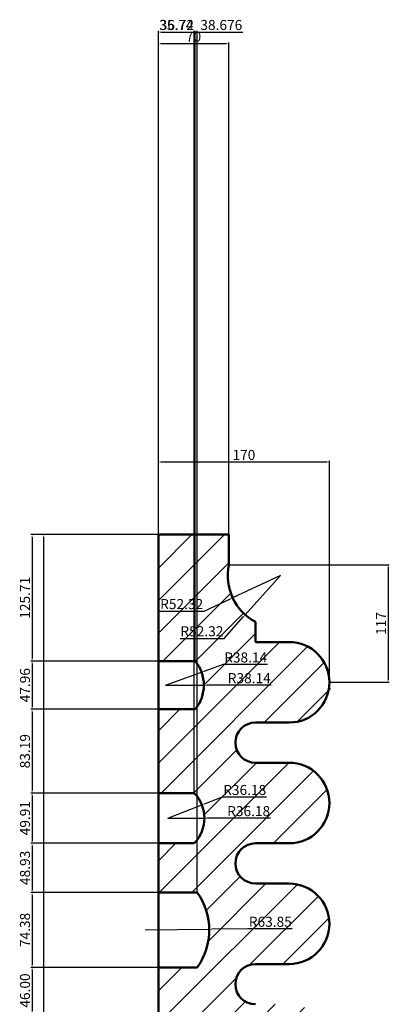
# Model space of a CAD drawing. Units: millimetres. Extents: x 1178 to 3717, y 924 to 2764.
# Tile 3 of 5: x 1208 to 1576, y 1785 to 2764. Entities that reach past the tile are written whole.
import ezdxf

# ---------------------------------------------------------------- set-up
doc = ezdxf.new("R2010")
doc.units = ezdxf.units.MM
for name, color, linetype, lineweight in [('M-DIMS', 2, 'Continuous', 25), ('M-HATC', 8, 'Continuous', 18), ('M-OUTL', 7, 'Continuous', 50)]:
    doc.layers.add(name, color=color, linetype=linetype, lineweight=lineweight)
doc.styles.get("Standard").update_dxf_attribs({"font": 'arial.ttf'})
doc.dimstyles.new('ISO-25', dxfattribs={"dimtxt": 10, "dimasz": 2.5, "dimexe": 1.25, "dimexo": 0.625, "dimtad": 1, "dimtoh": 1, "dimdec": 0, "dimtxsty": 'Standard', "dimcen": 2.5, "dimadec": 0, "dimazin": 0, "dimtfac": 1, "dimtdec": 0, "dimtmove": 0, "dimatfit": 3, "dimfxl": 1, "dimarcsym": 0})

# ---------------------------------------------------------------- blocks, each defined once
blk = doc.blocks.new('*D24')
at = {"layer": 'Defpoints', "color": 0, "transparency": 16777216}
for p in [(1516.06, 2324.34), (1346.06, 2252.21), (1516.06, 2099.53)]:
    blk.add_point(p, dxfattribs=at)
at = {"layer": 'M-DIMS', "color": 0, "lineweight": -2, "transparency": 16777216}
for p, q in [((1346.06, 2252.84), (1346.06, 2325.59)), ((1348.56, 2324.34), (1513.56, 2324.34)), ((1516.06, 2100.16), (1516.06, 2325.59))]:
    blk.add_line(p, q, dxfattribs=at)
at = {"layer": 'M-DIMS', "color": 0, "transparency": 16777216}
for points in [[(1348.56, 2324.76), (1348.56, 2323.93), (1346.06, 2324.34)], [(1513.56, 2324.76), (1513.56, 2323.93), (1516.06, 2324.34)]]:
    blk.add_solid(points, dxfattribs=at)
at = {"layer": 'M-DIMS', "color": 0, "transparency": 16777216, "insert": (1431.06, 2330.07), "char_height": 10, "attachment_point": 5}
blk.add_mtext('170', dxfattribs=at)
blk = doc.blocks.new('*D25')
at = {"layer": 'Defpoints', "color": 0, "transparency": 16777216}
for p in [(1416.06, 2222.21), (1516.07, 2105.43), (1574.3, 2105.43)]:
    blk.add_point(p, dxfattribs=at)
at = {"layer": 'M-DIMS', "color": 0, "lineweight": -2, "transparency": 16777216}
for p, q in [((1416.69, 2222.21), (1575.55, 2222.21)), ((1574.3, 2219.71), (1574.3, 2107.93)), ((1516.69, 2105.43), (1575.55, 2105.43))]:
    blk.add_line(p, q, dxfattribs=at)
at = {"layer": 'M-DIMS', "color": 0, "transparency": 16777216}
for points in [[(1573.89, 2219.71), (1574.72, 2219.71), (1574.3, 2222.21)], [(1573.89, 2107.93), (1574.72, 2107.93), (1574.3, 2105.43)]]:
    blk.add_solid(points, dxfattribs=at)
at = {"layer": 'M-DIMS', "color": 0, "transparency": 16777216, "insert": (1568.66, 2163.82), "char_height": 10, "attachment_point": 5, "rotation": 90}
blk.add_mtext('117', dxfattribs=at)
blk = doc.blocks.new('*D49')
at = {"layer": 'Defpoints', "color": 0, "transparency": 16777216}
for p in [(1346.06, 2252.21), (1232.06, 1051.02), (1346.06, 1051.02)]:
    blk.add_point(p, dxfattribs=at)
at = {"layer": 'M-DIMS', "color": 0, "lineweight": -2, "transparency": 16777216}
for p, q in [((1345.44, 2252.21), (1230.81, 2252.21)), ((1232.06, 2249.71), (1232.06, 1053.52)), ((1345.44, 1051.02), (1230.81, 1051.02))]:
    blk.add_line(p, q, dxfattribs=at)
at = {"layer": 'M-DIMS', "color": 0, "transparency": 16777216}
for points in [[(1231.64, 2249.71), (1232.48, 2249.71), (1232.06, 2252.21)], [(1231.64, 1053.52), (1232.48, 1053.52), (1232.06, 1051.02)]]:
    blk.add_solid(points, dxfattribs=at)
at = {"layer": 'M-DIMS', "color": 0, "transparency": 16777216, "insert": (1226.33, 1651.62), "char_height": 10, "attachment_point": 5, "rotation": 90}
blk.add_mtext('1201.2', dxfattribs=at)
blk = doc.blocks.new('*D50')
at = {"layer": 'Defpoints', "color": 0, "transparency": 16777216}
for p in [(1416.06, 2740.04), (1346.06, 2252.21), (1416.06, 2222.21)]:
    blk.add_point(p, dxfattribs=at)
at = {"layer": 'M-DIMS', "color": 0, "lineweight": -2, "transparency": 16777216}
for p, q in [((1346.06, 2252.84), (1346.06, 2741.29)), ((1348.56, 2740.04), (1413.56, 2740.04)), ((1416.06, 2222.84), (1416.06, 2741.29))]:
    blk.add_line(p, q, dxfattribs=at)
at = {"layer": 'M-DIMS', "color": 0, "transparency": 16777216}
for points in [[(1348.56, 2740.46), (1348.56, 2739.62), (1346.06, 2740.04)], [(1413.56, 2740.46), (1413.56, 2739.62), (1416.06, 2740.04)]]:
    blk.add_solid(points, dxfattribs=at)
at = {"layer": 'M-DIMS', "color": 0, "transparency": 16777216, "insert": (1381.06, 2745.77), "char_height": 10, "attachment_point": 5}
blk.add_mtext('70', dxfattribs=at)
blk = doc.blocks.new('*D60')
at = {"layer": 'Defpoints', "color": 0, "transparency": 16777216}
for p in [(1467.29, 2211.56), (1419.89, 2189.4)]:
    blk.add_point(p, dxfattribs=at)
at = {"layer": 'M-DIMS', "color": 0, "lineweight": -2, "transparency": 16777216}
for p, q in [((1467.29, 2211.56), (1419.89, 2189.4)), ((1391.46, 2176.1), (1417.63, 2188.34)), ((1347.62, 2176.1), (1391.46, 2176.1))]:
    blk.add_line(p, q, dxfattribs=at)
at = {"layer": 'M-DIMS', "color": 0, "transparency": 16777216}
blk.add_solid([(1417.45, 2188.72), (1417.81, 2187.96), (1419.89, 2189.4)], dxfattribs=at)
at = {"layer": 'M-DIMS', "color": 0, "transparency": 16777216, "insert": (1369.22, 2181.83), "char_height": 10, "attachment_point": 5}
blk.add_mtext('R52.32', dxfattribs=at)
blk = doc.blocks.new('*D63')
at = {"layer": 'Defpoints', "color": 0, "transparency": 16777216}
for p in [(1353.12, 2102.53), (1391.26, 2102.5)]:
    blk.add_point(p, dxfattribs=at)
at = {"layer": 'M-DIMS', "color": 0, "lineweight": -2, "transparency": 16777216}
for p, q in [((1353.12, 2102.53), (1391.26, 2102.5)), ((1414.14, 2102.48), (1393.76, 2102.5)), ((1458.04, 2102.48), (1414.14, 2102.48))]:
    blk.add_line(p, q, dxfattribs=at)
at = {"layer": 'M-DIMS', "color": 0, "transparency": 16777216}
blk.add_solid([(1393.76, 2102.91), (1393.76, 2102.08), (1391.26, 2102.5)], dxfattribs=at)
at = {"layer": 'M-DIMS', "color": 0, "transparency": 16777216, "insert": (1436.4, 2108.22), "char_height": 10, "attachment_point": 5}
blk.add_mtext('R38.14', dxfattribs=at)
blk = doc.blocks.new('*D64')
at = {"layer": 'Defpoints', "color": 0, "transparency": 16777216}
for p in [(1355.6, 1970.4), (1391.78, 1970.4)]:
    blk.add_point(p, dxfattribs=at)
at = {"layer": 'M-DIMS', "color": 0, "lineweight": -2, "transparency": 16777216}
for p, q in [((1355.6, 1970.4), (1391.78, 1970.4)), ((1413.49, 1970.4), (1394.28, 1970.4)), ((1457.45, 1970.4), (1413.49, 1970.4))]:
    blk.add_line(p, q, dxfattribs=at)
at = {"layer": 'M-DIMS', "color": 0, "transparency": 16777216}
blk.add_solid([(1394.28, 1970.82), (1394.28, 1969.98), (1391.78, 1970.4)], dxfattribs=at)
at = {"layer": 'M-DIMS', "color": 0, "transparency": 16777216, "insert": (1435.78, 1976.13), "char_height": 10, "attachment_point": 5}
blk.add_mtext('R36.18', dxfattribs=at)
blk = doc.blocks.new('*D72')
at = {"layer": 'Defpoints', "color": 0, "transparency": 16777216}
for p in [(1346.06, 2252.21), (1220.56, 2126.5), (1346.06, 2126.5)]:
    blk.add_point(p, dxfattribs=at)
at = {"layer": 'M-DIMS', "color": 0, "lineweight": -2, "transparency": 16777216}
for p, q in [((1345.44, 2252.21), (1219.31, 2252.21)), ((1220.56, 2249.71), (1220.56, 2129)), ((1345.44, 2126.5), (1219.31, 2126.5))]:
    blk.add_line(p, q, dxfattribs=at)
at = {"layer": 'M-DIMS', "color": 0, "transparency": 16777216}
for points in [[(1220.14, 2249.71), (1220.98, 2249.71), (1220.56, 2252.21)], [(1220.14, 2129), (1220.98, 2129), (1220.56, 2126.5)]]:
    blk.add_solid(points, dxfattribs=at)
at = {"layer": 'M-DIMS', "color": 0, "transparency": 16777216, "insert": (1214.83, 2189.36), "char_height": 10, "attachment_point": 5, "rotation": 90}
blk.add_mtext('125.71', dxfattribs=at)
blk = doc.blocks.new('*D73')
at = {"layer": 'Defpoints', "color": 0, "transparency": 16777216}
for p in [(1346.06, 2126.5), (1220.56, 2078.55), (1346.06, 2078.55)]:
    blk.add_point(p, dxfattribs=at)
at = {"layer": 'M-DIMS', "color": 0, "lineweight": -2, "transparency": 16777216}
for p, q in [((1345.44, 2126.5), (1219.31, 2126.5)), ((1220.56, 2124), (1220.56, 2081.05)), ((1345.44, 2078.55), (1219.31, 2078.55))]:
    blk.add_line(p, q, dxfattribs=at)
at = {"layer": 'M-DIMS', "color": 0, "transparency": 16777216}
for points in [[(1220.14, 2124), (1220.98, 2124), (1220.56, 2126.5)], [(1220.14, 2081.05), (1220.98, 2081.05), (1220.56, 2078.55)]]:
    blk.add_solid(points, dxfattribs=at)
at = {"layer": 'M-DIMS', "color": 0, "transparency": 16777216, "insert": (1214.83, 2102.53), "char_height": 10, "attachment_point": 5, "rotation": 90}
blk.add_mtext('47.96', dxfattribs=at)
blk = doc.blocks.new('*D74')
at = {"layer": 'Defpoints', "color": 0, "transparency": 16777216}
for p in [(1346.06, 2078.55), (1220.56, 1995.36), (1346.06, 1995.36)]:
    blk.add_point(p, dxfattribs=at)
at = {"layer": 'M-DIMS', "color": 0, "lineweight": -2, "transparency": 16777216}
for p, q in [((1345.44, 2078.55), (1219.31, 2078.55)), ((1220.56, 2076.05), (1220.56, 1997.86)), ((1345.44, 1995.36), (1219.31, 1995.36))]:
    blk.add_line(p, q, dxfattribs=at)
at = {"layer": 'M-DIMS', "color": 0, "transparency": 16777216}
for points in [[(1220.14, 2076.05), (1220.98, 2076.05), (1220.56, 2078.55)], [(1220.14, 1997.86), (1220.98, 1997.86), (1220.56, 1995.36)]]:
    blk.add_solid(points, dxfattribs=at)
at = {"layer": 'M-DIMS', "color": 0, "transparency": 16777216, "insert": (1214.83, 2036.95), "char_height": 10, "attachment_point": 5, "rotation": 90}
blk.add_mtext('83.19', dxfattribs=at)
blk = doc.blocks.new('*D75')
at = {"layer": 'Defpoints', "color": 0, "transparency": 16777216}
for p in [(1346.06, 1995.36), (1220.56, 1945.45), (1346.06, 1945.45)]:
    blk.add_point(p, dxfattribs=at)
at = {"layer": 'M-DIMS', "color": 0, "lineweight": -2, "transparency": 16777216}
for p, q in [((1345.44, 1995.36), (1219.31, 1995.36)), ((1220.56, 1992.86), (1220.56, 1947.95)), ((1345.44, 1945.45), (1219.31, 1945.45))]:
    blk.add_line(p, q, dxfattribs=at)
at = {"layer": 'M-DIMS', "color": 0, "transparency": 16777216}
for points in [[(1220.14, 1992.86), (1220.98, 1992.86), (1220.56, 1995.36)], [(1220.14, 1947.95), (1220.98, 1947.95), (1220.56, 1945.45)]]:
    blk.add_solid(points, dxfattribs=at)
at = {"layer": 'M-DIMS', "color": 0, "transparency": 16777216, "insert": (1214.83, 1970.4), "char_height": 10, "attachment_point": 5, "rotation": 90}
blk.add_mtext('49.91', dxfattribs=at)
blk = doc.blocks.new('*D76')
at = {"layer": 'Defpoints', "color": 0, "transparency": 16777216}
for p in [(1346.06, 1945.45), (1220.56, 1896.51), (1346.06, 1896.51)]:
    blk.add_point(p, dxfattribs=at)
at = {"layer": 'M-DIMS', "color": 0, "lineweight": -2, "transparency": 16777216}
for p, q in [((1345.44, 1945.45), (1219.31, 1945.45)), ((1220.56, 1942.95), (1220.56, 1899.01)), ((1345.44, 1896.51), (1219.31, 1896.51))]:
    blk.add_line(p, q, dxfattribs=at)
at = {"layer": 'M-DIMS', "color": 0, "transparency": 16777216}
for points in [[(1220.14, 1942.95), (1220.98, 1942.95), (1220.56, 1945.45)], [(1220.14, 1899.01), (1220.98, 1899.01), (1220.56, 1896.51)]]:
    blk.add_solid(points, dxfattribs=at)
at = {"layer": 'M-DIMS', "color": 0, "transparency": 16777216, "insert": (1214.83, 1920.98), "char_height": 10, "attachment_point": 5, "rotation": 90}
blk.add_mtext('48.93', dxfattribs=at)
blk = doc.blocks.new('*D77')
at = {"layer": 'Defpoints', "color": 0, "transparency": 16777216}
for p in [(1346.06, 1896.51), (1220.56, 1822.13), (1346.06, 1822.13)]:
    blk.add_point(p, dxfattribs=at)
at = {"layer": 'M-DIMS', "color": 0, "lineweight": -2, "transparency": 16777216}
for p, q in [((1345.44, 1896.51), (1219.31, 1896.51)), ((1220.56, 1894.01), (1220.56, 1824.63)), ((1345.44, 1822.13), (1219.31, 1822.13))]:
    blk.add_line(p, q, dxfattribs=at)
at = {"layer": 'M-DIMS', "color": 0, "transparency": 16777216}
for points in [[(1220.14, 1894.01), (1220.98, 1894.01), (1220.56, 1896.51)], [(1220.14, 1824.63), (1220.98, 1824.63), (1220.56, 1822.13)]]:
    blk.add_solid(points, dxfattribs=at)
at = {"layer": 'M-DIMS', "color": 0, "transparency": 16777216, "insert": (1214.83, 1859.32), "char_height": 10, "attachment_point": 5, "rotation": 90}
blk.add_mtext('74.38', dxfattribs=at)
blk = doc.blocks.new('*D78')
at = {"layer": 'Defpoints', "color": 0, "transparency": 16777216}
for p in [(1346.06, 1822.13), (1220.56, 1776.13), (1346.06, 1776.13)]:
    blk.add_point(p, dxfattribs=at)
at = {"layer": 'M-DIMS', "color": 0, "lineweight": -2, "transparency": 16777216}
for p, q in [((1345.44, 1822.13), (1219.31, 1822.13)), ((1220.56, 1819.63), (1220.56, 1778.63)), ((1345.44, 1776.13), (1219.31, 1776.13))]:
    blk.add_line(p, q, dxfattribs=at)
at = {"layer": 'M-DIMS', "color": 0, "transparency": 16777216}
for points in [[(1220.14, 1819.63), (1220.98, 1819.63), (1220.56, 1822.13)], [(1220.14, 1778.63), (1220.98, 1778.63), (1220.56, 1776.13)]]:
    blk.add_solid(points, dxfattribs=at)
at = {"layer": 'M-DIMS', "color": 0, "transparency": 16777216, "insert": (1214.83, 1799.13), "char_height": 10, "attachment_point": 5, "rotation": 90}
blk.add_mtext('46.00', dxfattribs=at)
blk = doc.blocks.new('*D90')
at = {"layer": 'Defpoints', "color": 0, "transparency": 16777216}
for p in [(1382.78, 2751.54), (1346.06, 2126.5), (1382.78, 2126.5)]:
    blk.add_point(p, dxfattribs=at)
at = {"layer": 'M-DIMS', "color": 0, "lineweight": -2, "transparency": 16777216}
for p, q in [((1346.06, 2127.13), (1346.06, 2752.79)), ((1348.56, 2751.54), (1380.28, 2751.54)), ((1382.78, 2127.13), (1382.78, 2752.79))]:
    blk.add_line(p, q, dxfattribs=at)
at = {"layer": 'M-DIMS', "color": 0, "transparency": 16777216}
for points in [[(1348.56, 2751.96), (1348.56, 2751.12), (1346.06, 2751.54)], [(1380.28, 2751.96), (1380.28, 2751.12), (1382.78, 2751.54)]]:
    blk.add_solid(points, dxfattribs=at)
at = {"layer": 'M-DIMS', "color": 0, "transparency": 16777216, "insert": (1364.42, 2757.28), "char_height": 10, "attachment_point": 5}
blk.add_mtext('36.72', dxfattribs=at)
blk = doc.blocks.new('*D91')
at = {"layer": 'Defpoints', "color": 0, "transparency": 16777216}
for p in [(1381.8, 2751.54), (1346.06, 1995.36), (1381.8, 1995.36)]:
    blk.add_point(p, dxfattribs=at)
at = {"layer": 'M-DIMS', "color": 0, "lineweight": -2, "transparency": 16777216}
for p, q in [((1346.06, 1995.99), (1346.06, 2752.79)), ((1348.56, 2751.54), (1379.3, 2751.54)), ((1381.8, 1995.99), (1381.8, 2752.79))]:
    blk.add_line(p, q, dxfattribs=at)
at = {"layer": 'M-DIMS', "color": 0, "transparency": 16777216}
for points in [[(1348.56, 2751.96), (1348.56, 2751.12), (1346.06, 2751.54)], [(1379.3, 2751.96), (1379.3, 2751.12), (1381.8, 2751.54)]]:
    blk.add_solid(points, dxfattribs=at)
at = {"layer": 'M-DIMS', "color": 0, "transparency": 16777216, "insert": (1363.93, 2757.28), "char_height": 10, "attachment_point": 5}
blk.add_mtext('35.74', dxfattribs=at)
blk = doc.blocks.new('*D92')
at = {"layer": 'Defpoints', "color": 0, "transparency": 16777216}
for p in [(1384.74, 2751.54), (1346.06, 1896.51), (1384.74, 1896.51)]:
    blk.add_point(p, dxfattribs=at)
at = {"layer": 'M-DIMS', "color": 0, "lineweight": -2, "transparency": 16777216}
for p, q in [((1346.06, 1897.14), (1346.06, 2752.79)), ((1348.56, 2751.54), (1382.24, 2751.54)), ((1384.74, 1897.14), (1384.74, 2752.79)), ((1384.74, 2751.54), (1429.99, 2751.54))]:
    blk.add_line(p, q, dxfattribs=at)
at = {"layer": 'M-DIMS', "color": 0, "transparency": 16777216}
for points in [[(1348.56, 2751.96), (1348.56, 2751.12), (1346.06, 2751.54)], [(1382.24, 2751.96), (1382.24, 2751.12), (1384.74, 2751.54)]]:
    blk.add_solid(points, dxfattribs=at)
at = {"layer": 'M-DIMS', "color": 0, "transparency": 16777216, "insert": (1408.61, 2757.28), "char_height": 10, "attachment_point": 5}
blk.add_mtext('38.676', dxfattribs=at)
blk = doc.blocks.new('*D102')
at = {"layer": 'Defpoints', "color": 0, "transparency": 16777216}
for p in [(1467.29, 2211.56), (1432.46, 2172.52)]:
    blk.add_point(p, dxfattribs=at)
at = {"layer": 'M-DIMS', "color": 0, "lineweight": -2, "transparency": 16777216}
for p, q in [((1467.29, 2211.56), (1432.46, 2172.52)), ((1411.56, 2149.09), (1430.8, 2170.65)), ((1367.72, 2149.09), (1411.56, 2149.09))]:
    blk.add_line(p, q, dxfattribs=at)
at = {"layer": 'M-DIMS', "color": 0, "transparency": 16777216}
blk.add_solid([(1430.49, 2170.93), (1431.11, 2170.37), (1432.46, 2172.52)], dxfattribs=at)
at = {"layer": 'M-DIMS', "color": 0, "transparency": 16777216, "insert": (1389.33, 2154.82), "char_height": 10, "attachment_point": 5}
blk.add_mtext('R52.32', dxfattribs=at)
blk = doc.blocks.new('*D103')
at = {"layer": 'Defpoints', "color": 0, "transparency": 16777216}
for p in [(1389.03, 2115.37), (1353.12, 2102.53)]:
    blk.add_point(p, dxfattribs=at)
at = {"layer": 'M-DIMS', "color": 0, "lineweight": -2, "transparency": 16777216}
for p, q in [((1353.12, 2102.53), (1389.03, 2115.37)), ((1410.58, 2123.07), (1391.38, 2116.21)), ((1454.48, 2123.07), (1410.58, 2123.07))]:
    blk.add_line(p, q, dxfattribs=at)
at = {"layer": 'M-DIMS', "color": 0, "transparency": 16777216}
blk.add_solid([(1391.24, 2116.6), (1391.53, 2115.82), (1389.03, 2115.37)], dxfattribs=at)
at = {"layer": 'M-DIMS', "color": 0, "transparency": 16777216, "insert": (1432.84, 2128.81), "char_height": 10, "attachment_point": 5}
blk.add_mtext('R38.14', dxfattribs=at)
blk = doc.blocks.new('*D104')
at = {"layer": 'Defpoints', "color": 0, "transparency": 16777216}
for p in [(1389.32, 1983.51), (1355.6, 1970.4)]:
    blk.add_point(p, dxfattribs=at)
at = {"layer": 'M-DIMS', "color": 0, "lineweight": -2, "transparency": 16777216}
for p, q in [((1409.56, 1991.38), (1391.65, 1984.42)), ((1453.52, 1991.38), (1409.56, 1991.38)), ((1355.6, 1970.4), (1389.32, 1983.51))]:
    blk.add_line(p, q, dxfattribs=at)
at = {"layer": 'M-DIMS', "color": 0, "transparency": 16777216}
blk.add_solid([(1391.5, 1984.81), (1391.8, 1984.03), (1389.32, 1983.51)], dxfattribs=at)
at = {"layer": 'M-DIMS', "color": 0, "transparency": 16777216, "insert": (1431.85, 1997.11), "char_height": 10, "attachment_point": 5}
blk.add_mtext('R36.18', dxfattribs=at)
blk = doc.blocks.new('*D105')
at = {"layer": 'Defpoints', "color": 0, "transparency": 16777216}
for p in [(1332.83, 1859.32), (1396.68, 1860)]:
    blk.add_point(p, dxfattribs=at)
at = {"layer": 'M-DIMS', "color": 0, "lineweight": -2, "transparency": 16777216}
for p, q in [((1332.83, 1859.32), (1396.68, 1860)), ((1434.99, 1860.41), (1399.18, 1860.03)), ((1479.01, 1860.41), (1434.99, 1860.41))]:
    blk.add_line(p, q, dxfattribs=at)
at = {"layer": 'M-DIMS', "color": 0, "transparency": 16777216}
blk.add_solid([(1399.18, 1860.44), (1399.19, 1859.61), (1396.68, 1860)], dxfattribs=at)
at = {"layer": 'M-DIMS', "color": 0, "transparency": 16777216, "insert": (1457.31, 1866.14), "char_height": 10, "attachment_point": 5}
blk.add_mtext('R63.85', dxfattribs=at)

msp = doc.modelspace()

# ---------------------------------------------------------------- hatches: boundary and pattern name
at = {"layer": 'M-HATC'}
h = msp.add_hatch(dxfattribs=at)
h.set_pattern_fill('ANSI31', color=256, scale=7.2)
h.paths.add_polyline_path([(1476.0659, 2145.4337), (1442.5959, 2145.4337), (1442.5959, 2165.4337, -0.33256542), (1416.0609, 2222.2134), (1416.0609, 2252.2134), (1346.0609, 2252.2134), (1346.0609, 2126.505), (1382.7778, 2126.505, -0.35365424), (1382.7778, 2078.5493), (1346.0609, 2078.5493), (1346.0609, 1995.3607), (1381.7982, 1995.3607, -0.40006542), (1381.7982, 1945.4476), (1346.0609, 1945.4476), (1346.0609, 1896.5132), (1384.7368, 1896.5132, -0.32128688), (1384.7368, 1822.1329), (1346.0609, 1822.1329), (1346.0609, 1776.1345), (1382.7778, 1776.1345, -0.38644482), (1382.7778, 1700.7755), (1346.0609, 1700.7755), (1346.0609, 1664.1898), (1388.6514, 1664.1898, -0.35526713), (1388.6514, 1580.0226), (1346.0609, 1580.0226), (1346.0609, 1549.6833), (1381.7946, 1549.6833, -0.46058316), (1381.7946, 1469.4308), (1346.0609, 1469.4308), (1346.0609, 1430.0146), (1385.7005, 1430.0146, -0.34111668), (1385.7005, 1349.7622), (1346.0609, 1349.7622), (1346.0609, 1313.5507), (1384.7209, 1313.5507, -0.34142199), (1384.7209, 1222.5327), (1346.0609, 1222.5327), (1346.0609, 1181.0495), (1382.7495, 1181.0495, -0.3326402), (1382.7495, 1116.456), (1346.0609, 1116.456), (1346.0609, 1051.0224), (1416.0609, 1051.0224), (1416.0609, 1081.0224, -0.31910694), (1453.0456, 1105.4337), (1476.0609, 1105.4337, 1), (1476.0609, 1185.4337), (1442.5959, 1185.4337, -1), (1442.5959, 1225.4337), (1476.0659, 1225.4337, 1), (1476.0659, 1305.4337), (1442.5959, 1305.4337, -1), (1442.5959, 1345.4337), (1476.0659, 1345.4337, 1), (1476.0659, 1425.4337), (1442.5959, 1425.4337, -1), (1442.5959, 1465.4337), (1476.0659, 1465.4337, 1), (1476.0659, 1545.4337), (1442.5959, 1545.4337, -1), (1442.5959, 1585.4337), (1476.0659, 1585.4337, 1), (1476.0659, 1665.4337), (1442.5959, 1665.4337, -1), (1442.5959, 1705.4337), (1476.0659, 1705.4337, 1), (1476.0659, 1785.4337), (1442.5959, 1785.4337, -1), (1442.5959, 1825.4337), (1476.0659, 1825.4337, 1), (1476.0659, 1905.4337), (1442.5959, 1905.4337, -1), (1442.5959, 1945.4337), (1476.0659, 1945.4337, 1), (1476.0659, 2025.4337), (1442.5959, 2025.4337, -1), (1442.5959, 2065.4337), (1476.0659, 2065.4337, 1)])

# ---------------------------------------------------------------- linework, layer by layer
at = {"layer": 'M-OUTL'}
for p, q in [((1346.0609, 2252.2134), (1346.0609, 1051.0224)), ((1346.0609, 2252.2134), (1416.0609, 2252.2134)), ((1416.0609, 2252.2134), (1416.0609, 2222.2134)), ((1442.5959, 2145.4337), (1442.5959, 2165.4337)), ((1476.0659, 2145.4337), (1442.5959, 2145.4337)), ((1346.0609, 2126.505), (1382.7778, 2126.505)), ((1382.7778, 2078.5493), (1346.0609, 2078.5493)), ((1442.5959, 2065.4337), (1476.0659, 2065.4337)), ((1476.0659, 2025.4337), (1442.5959, 2025.4337)), ((1346.0609, 1995.3607), (1381.7982, 1995.3607)), ((1381.7982, 1945.4476), (1346.0609, 1945.4476)), ((1442.5959, 1945.4337), (1476.0659, 1945.4337)), ((1476.0659, 1905.4337), (1442.5959, 1905.4337)), ((1346.0609, 1896.5132), (1384.7368, 1896.5132)), ((1384.7368, 1822.1329), (1346.0609, 1822.1329)), ((1442.5959, 1825.4337), (1476.0659, 1825.4337))]:
    msp.add_line(p, q, dxfattribs=at)
for centre, radius, start, end in [((1467.2907, 2211.5646), 52.3249, 168.2574937, 241.8388584), ((1476.0659, 2105.4337), 40, 270, 90), ((1353.1175, 2102.5271), 38.1401, 321.0472867, 38.9527133), ((1476.0659, 2098.9037), 40, 359.09819, 0.90181), ((1442.5959, 2045.4337), 20, 90, 270), ((1476.0659, 1985.4337), 40, 270, 90), ((1355.5997, 1970.4042), 36.1827, 316.3907183, 43.6092817), ((1442.5959, 1925.4337), 20, 90, 270), ((1476.0659, 1865.4337), 40, 270, 90), ((1332.8343, 1859.323), 63.8512, 324.3769389, 35.6230611), ((1442.5959, 1805.4337), 20, 90, 270)]:
    msp.add_arc(centre, radius, start, end, dxfattribs=at)

# ---------------------------------------------------------------- dimensions: what is measured, and where the dimension line sits
at = {"layer": 'M-DIMS'}
for base, p1, p2, override, picture, middle in [((1382.7778, 2751.5416), (1346.0609, 2126.505), (1382.7778, 2126.505), {"dimdec": 2, "dimlfac": 1, "dimrnd": 0, "dimzin": 0, "dimdsep": 46, "dimlunit": 2}, '*D90', (1364.4193, 2757.2757)), ((1381.7982, 2751.5416), (1346.0609, 1995.3607), (1381.7982, 1995.3607), {"dimdec": 2, "dimlfac": 1, "dimrnd": 0, "dimzin": 0, "dimdsep": 46, "dimlunit": 2}, '*D91', (1363.9296, 2757.2757)), ((1384.7368, 2751.5416), (1346.0609, 1896.5132), (1384.7368, 1896.5132), {"dimdec": 3, "dimlfac": 1, "dimrnd": 0, "dimzin": 0, "dimdsep": 46, "dimlunit": 2}, '*D92', (1408.6122, 2757.2757)), ((1416.0609, 2740.0416), (1346.0609, 2252.2134), (1416.0609, 2222.2134), {"dimdec": 0, "dimlfac": 1, "dimrnd": 0, "dimzin": 0, "dimdsep": 46, "dimlunit": 2}, '*D50', (1381.0609, 2745.7723)), ((1516.0609, 2324.3428), (1346.0609, 2252.2134), (1516.0609, 2099.5333), {"dimclrd": 0, "dimclre": 0, "dimclrt": 0}, '*D24', (1431.0609, 2330.0735))]:
    dim = msp.add_linear_dim(base=base, p1=p1, p2=p2, dimstyle='ISO-25', override=override, dxfattribs=at)
    dim.commit()
    dim.dimension.update_dxf_attribs({"geometry": picture, "text_midpoint": middle})
for base, p1, p2, override, picture, middle in [((1220.5609, 2126.505), (1346.0609, 2252.2134), (1346.0609, 2126.505), {"dimdec": 2, "dimlfac": 1, "dimrnd": 0, "dimzin": 0, "dimdsep": 46, "dimlunit": 2}, '*D72', (1214.8302, 2189.3592)), ((1232.0609, 1051.0224), (1346.0609, 2252.2134), (1346.0609, 1051.0224), {"dimdec": 1, "dimlfac": 1, "dimrnd": 0, "dimzin": 0, "dimdsep": 46, "dimlunit": 2}, '*D49', (1226.3302, 1651.6179)), ((1574.3026, 2105.4337), (1416.0609, 2222.2134), (1516.0659, 2105.4337), {"dimclrd": 0, "dimclre": 0, "dimclrt": 0}, '*D25', (1568.6571, 2163.8236)), ((1220.5609, 2078.5493), (1346.0609, 2126.505), (1346.0609, 2078.5493), {"dimdec": 2, "dimlfac": 1, "dimrnd": 0, "dimzin": 0, "dimdsep": 46, "dimlunit": 2}, '*D73', (1214.8302, 2102.5271)), ((1220.5609, 1995.3607), (1346.0609, 2078.5493), (1346.0609, 1995.3607), {"dimdec": 2, "dimlfac": 1, "dimrnd": 0, "dimzin": 0, "dimdsep": 46, "dimlunit": 2}, '*D74', (1214.8268, 2036.955)), ((1220.5609, 1945.4476), (1346.0609, 1995.3607), (1346.0609, 1945.4476), {"dimdec": 2, "dimlfac": 1, "dimrnd": 0, "dimzin": 0, "dimdsep": 46, "dimlunit": 2}, '*D75', (1214.8302, 1970.4042)), ((1220.5609, 1896.5132), (1346.0609, 1945.4476), (1346.0609, 1896.5132), {"dimdec": 2, "dimlfac": 1, "dimrnd": 0, "dimzin": 0, "dimdsep": 46, "dimlunit": 2}, '*D76', (1214.8268, 1920.9804)), ((1220.5609, 1822.1329), (1346.0609, 1896.5132), (1346.0609, 1822.1329), {"dimdec": 2, "dimlfac": 1, "dimrnd": 0, "dimzin": 0, "dimdsep": 46, "dimlunit": 2}, '*D77', (1214.8268, 1859.323)), ((1220.5609, 1776.1345), (1346.0609, 1822.1329), (1346.0609, 1776.1345), {"dimdec": 2, "dimlfac": 1, "dimrnd": 0, "dimzin": 0, "dimdsep": 46, "dimlunit": 2}, '*D78', (1214.8302, 1799.1337))]:
    dim = msp.add_linear_dim(base=base, p1=p1, p2=p2, angle=90, dimstyle='ISO-25', override=override, dxfattribs=at)
    dim.commit()
    dim.dimension.update_dxf_attribs({"geometry": picture, "text_midpoint": middle})
for center, mpoint, picture, middle in [((1467.2907, 2211.5646), (1419.8936, 2189.397), '*D60', (1369.2239, 2176.0964)), ((1467.2907, 2211.5646), (1432.4606, 2172.5164), '*D102', (1389.3312, 2149.0875)), ((1353.1175, 2102.5271), (1389.0308, 2115.3686), '*D103', (1432.8409, 2123.0735)), ((1353.1175, 2102.5271), (1391.2576, 2102.5), '*D63', (1414.1417, 2102.4838)), ((1355.5997, 1970.4042), (1389.3237, 1983.5146), '*D104', (1431.8509, 1991.3809)), ((1355.5997, 1970.4042), (1391.7825, 1970.4), '*D64', (1413.4921, 1970.3975)), ((1332.8343, 1859.323), (1396.682, 1860.0009), '*D105', (1434.9905, 1860.4076))]:
    dim = msp.add_radius_dim(center=center, mpoint=mpoint, dimstyle='ISO-25', override={"dimdec": 2, "dimlfac": 1, "dimrnd": 0, "dimzin": 0, "dimdsep": 46, "dimlunit": 2}, dxfattribs=at)
    dim.commit()
    dim.dimension.update_dxf_attribs({"geometry": picture, "text_midpoint": middle, "dimtype": 164})

doc.saveas('drawing.dxf')
